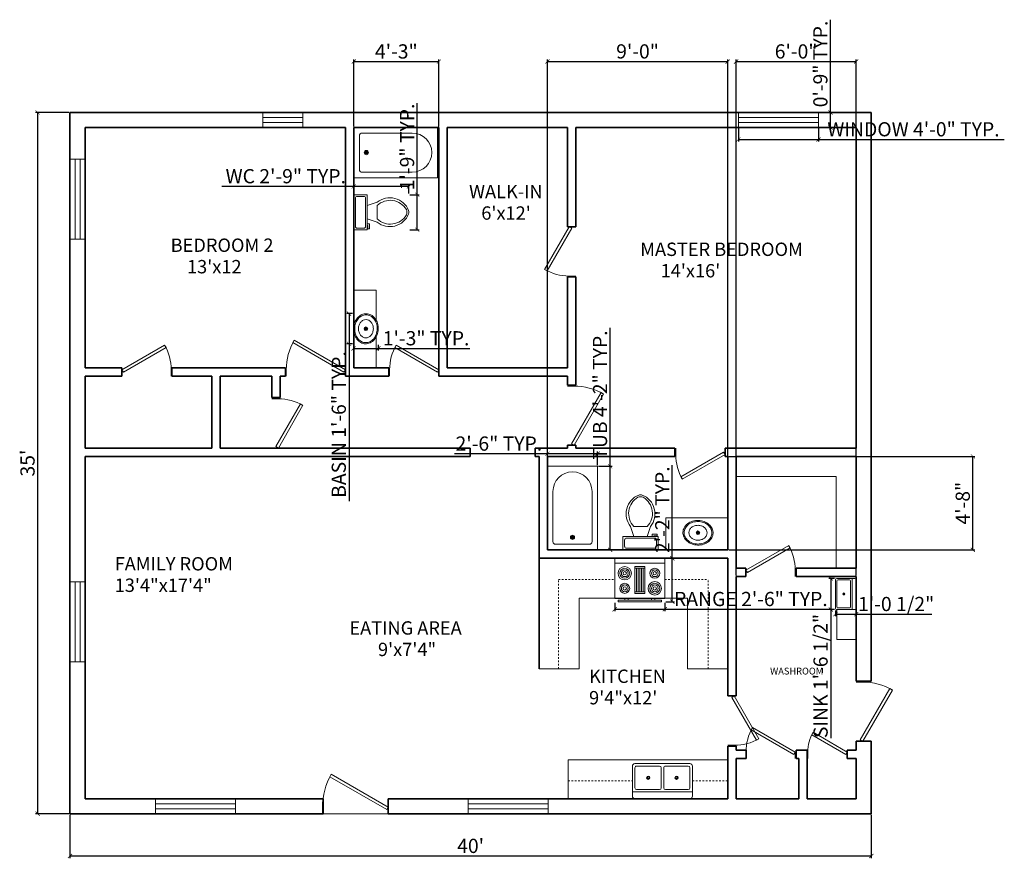
# Model space of a CAD drawing. Units: inches. Extents: x 3799 to 20199, y 1682 to 8087.
# Tile 25 of 30: x 17831 to 18421, y 2751 to 3254. Entities that reach past the tile are written whole.
import ezdxf

# ---------------------------------------------------------------- set-up
doc = ezdxf.new("R2010")
doc.units = ezdxf.units.IN
doc.linetypes.add('JIS_02_1.0', pattern=[2, 1, -1])
for name, color, linetype, lineweight in [('A-ANNO-DIMS', 2, 'Continuous', 18), ('A-AREA-IDEN', 7, 'Continuous', 18), ('A-DOOR', 3, 'Continuous', 18), ('A-EQPM', 9, 'Continuous', 18), ('A-FLOR-CASE', 32, 'Continuous', 18), ('A-FLOR-CASE-OVHD', 32, 'JIS_02_1.0', 13), ('A-FLOR-FIXT', 9, 'Continuous', 18), ('A-FURN', 8, 'Continuous', 18), ('A-GLAZ', 152, 'Continuous', 18), ('A-WALL', 7, 'Continuous', 35)]:
    doc.layers.add(name, color=color, linetype=linetype, lineweight=lineweight)
doc.styles.get("Standard").update_dxf_attribs({"font": 'arial.ttf'})
doc.dimstyles.new('ISO-25', dxfattribs={"dimtxt": 8.5, "dimasz": 2.5, "dimexe": 1.25, "dimexo": 0.625, "dimtad": 1, "dimdec": 0, "dimlunit": 3, "dimtxsty": 'Standard', "dimblk": 'ARCHTICK', "dimcen": 2.5, "dimadec": 0, "dimazin": 0, "dimtfac": 1, "dimtdec": 0, "dimtmove": 0, "dimatfit": 3, "dimfxl": 1, "dimarcsym": 0})

# ---------------------------------------------------------------- blocks, each defined once
blk = doc.blocks.new('*U134')
for p, q in [((0, 0), (0, -100)), ((750, 0), (750, -100))]:
    blk.add_line(p, q)
blk.add_lwpolyline([(0, 0), (650, 375), (671, 337), (22, -38)], close=True)
blk.add_arc((0, 0), 750, 0, 30)
blk = doc.blocks.new('*U135')
for p, q in [((0, 0), (0, -100)), ((-900, 0), (-900, -100))]:
    blk.add_line(p, q)
blk.add_lwpolyline([(0, 0), (-779, 450), (-801, 412), (-22, -38)], close=True)
blk.add_arc((0, 0), 900, 150, 180)
blk = doc.blocks.new('*U136')
for p, q in [((-750, 0), (-750, -100)), ((0, 0), (0, -100))]:
    blk.add_line(p, q)
blk.add_lwpolyline([(0, 0), (-650, 375), (-671, 337), (-22, -38)], close=True)
blk.add_arc((0, 0), 750, 150, 180)
blk = doc.blocks.new('*U141')
for p, q in [((0, 0), (0, -100)), ((750, 0), (750, -100))]:
    blk.add_line(p, q)
blk.add_lwpolyline([(0, 0), (650, 375), (671, 337), (22, -38)], close=True)
blk.add_arc((0, 0), 750, 0, 30)
blk = doc.blocks.new('*U138')
for p, q in [((-750, 0), (-750, 100)), ((0, 0), (0, 100))]:
    blk.add_line(p, q)
blk.add_lwpolyline([(0, 0), (-650, -375), (-671, -337), (-22, 38)], close=True)
blk.add_arc((0, 0), 750, 180, 210)
blk = doc.blocks.new('*U139')
for p, q in [((0, 0), (0, -100)), ((-1000, 0), (-1000, -100))]:
    blk.add_line(p, q)
blk.add_lwpolyline([(0, 0), (-866, 500), (-888, 462), (-22, -38)], close=True)
blk.add_arc((0, 0), 1000, 150, 180)
blk = doc.blocks.new('*U140')
for p, q in [((-750, 0), (-750, -100)), ((0, 0), (0, -100))]:
    blk.add_line(p, q)
blk.add_lwpolyline([(0, 0), (-650, 375), (-671, 337), (-22, -38)], close=True)
blk.add_arc((0, 0), 750, 150, 180)
blk = doc.blocks.new('*U142')
for p, q in [((-600, 0), (-600, -100)), ((0, 0), (0, -100))]:
    blk.add_line(p, q)
blk.add_lwpolyline([(0, 0), (-520, 300), (-541, 262), (-22, -38)], close=True)
blk.add_arc((0, 0), 600, 150, 180)
blk = doc.blocks.new('Bath Tub - 26 x 60 in.')
for p, q in [((8, -18), (10, -18)), ((9, -17), (9, -19))]:
    blk.add_line(p, q)
blk.add_lwpolyline([(0, -36), (0, 0), (60, 0), (60, -36)], close=True)
for points in [[(4, -30), (4, -6)], [(6, -4), (42, -4)], [(42, -32), (6, -32)]]:
    blk.add_lwpolyline(points)
for radius in [1.5, 1]:
    blk.add_circle((9, -18), radius)
for centre, radius, start, end in [((5.75, -5.75), 1.77, 81.8699, 188.1301), ((42, -18), 14, 270, 90), ((5.75, -30.25), 1.77, 171.8699, 278.1301)]:
    blk.add_arc(centre, radius, start, end)
blk = doc.blocks.new('Toilet - top')
for p, q in [((9.5, -6), (9.5, -2)), ((-10, -8.5), (-8, -8.5)), ((-10, -9.5), (-10, -8.5)), ((-7, -9.5), (-10, -9.5)), ((-8, -8.5), (-8, -8)), ((-7, -8), (-7, -9.5)), ((-4, -8), (-6, -14)), ((4, -8), (6, -14)), ((4, -14), (-4, -14))]:
    blk.add_line(p, q)
blk.add_lwpolyline([(10.5, -8), (10.5, 0), (-10.5, 0), (-10.5, -8)], close=True)
for points in [[(-9.5, -2), (-9.5, -6)], [(8.5, -1), (-8.5, -1)], [(-8.5, -7), (8.5, -7)]]:
    blk.add_lwpolyline(points)
for centre, radius, start, end in [((-8.62, -1.88), 0.884, 81.8699, 188.1301), ((8.62, -1.88), 0.884, 351.8699, 98.1301), ((-8.62, -6.12), 0.884, 171.8699, 278.1301), ((8.62, -6.12), 0.884, 261.8699, 8.1301), ((3.52, -21.58), 12.17, 141.46911, 247.97143), ((4.2, -21.82), 11.33, 136.36773, 238.94682), ((-3.52, -21.58), 12.17, 292.02843, 38.53071), ((-4.2, -21.82), 11.33, 301.05301, 43.63209), ((0, -27.88), 4, 245.73182, 294.26817), ((0, -29), 4, 254.86053, 285.13947)]:
    blk.add_arc(centre, radius, start, end)
blk = doc.blocks.new('Sink - Oval top')
for p, q in [((-1, 0), (1, 0)), ((0, 1), (0, -1))]:
    blk.add_line(p, q)
for points in [[(-12.23, 0.39, 0.117634), (-11.46, -3.36, 0.104469), (-8.88, -6.8, 0.090016), (-5.08, -9.07, 0.08192), (-0.32, -10.02, 0.08192), (4.49, -9.38, 0.090016), (8.42, -7.36, 0.104469), (11.22, -4.09, 0.117634), (12.23, -0.39, 0.117634), (11.46, 3.36, 0.104469), (8.88, 6.8, 0.090016), (5.08, 9.07, 0.08192), (0.32, 10.02, 0.08192), (-4.49, 9.38, 0.090016), (-8.42, 7.36, 0.104469), (-11.22, 4.09, 0.117634)], [(-11.29, 0.16, 0.118622), (-10.52, -3.25, 0.104678), (-8.07, -6.36, 0.089562), (-4.54, -8.37, 0.081185), (-0.13, -9.15, 0.081185), (4.3, -8.49, 0.089562), (7.89, -6.58, 0.104678), (10.42, -3.55, 0.118622), (11.29, -0.16, 0.118622), (10.52, 3.25, 0.104678), (8.07, 6.36, 0.089562), (4.54, 8.37, 0.081185), (0.13, 9.15, 0.081185), (-4.3, 8.49, 0.089562), (-7.89, 6.58, 0.104678), (-10.42, 3.55, 0.118622)], [(-7.42, 0.08, 0.118283), (-6.91, -2.17, 0.104607), (-5.29, -4.21, 0.089718), (-2.97, -5.53, 0.081436), (-0.07, -6.04, 0.081436), (2.84, -5.59, 0.089718), (5.2, -4.33, 0.104607), (6.86, -2.32, 0.118283), (7.42, -0.08, 0.118283), (6.91, 2.17, 0.104607), (5.29, 4.21, 0.089718), (2.97, 5.53, 0.081436), (0.07, 6.04, 0.081436), (-2.84, 5.59, 0.089718), (-5.2, 4.33, 0.104607), (-6.86, 2.32, 0.118283)]]:
    blk.add_lwpolyline(points, format="xyb", close=True)
for radius in [1.5, 1]:
    blk.add_circle((0, 0), radius)
blk = doc.blocks.new('Range-Oven - 30 in top')
for p, q in [((0, -3), (30, -3)), ((12, -6), (18, -6)), ((13, -20), (13, -6)), ((14, -6), (14, -20)), ((15, -20), (15, -6)), ((16, -6), (16, -20)), ((17, -20), (17, -6)), ((18, -20), (12, -20)), ((6, -24), (6, -25)), ((8, -25), (8, -24)), ((22, -25), (22, -24)), ((24, -24), (24, -25))]:
    blk.add_line(p, q)
for points in [[(0, -24), (0, 0), (30, 0), (30, -24)], [(12, -21), (12, -5), (18, -5), (18, -21)], [(2, -26), (2, -25), (28, -25), (28, -26)]]:
    blk.add_lwpolyline(points, close=True)
for centre, radius in [((6, -9), 4), ((6, -9), 3), ((6, -9), 2), ((6, -9), 1), ((24, -9), 3), ((24, -9), 2), ((24, -9), 1), ((6, -18), 3), ((6, -18), 2), ((6, -18), 1), ((24, -18), 4), ((24, -18), 3), ((24, -18), 2), ((24, -18), 1)]:
    blk.add_circle(centre, radius)
blk = doc.blocks.new('Sink-double - 36 in top')
for p, q in [((-18, -4), (18, -4)), ((-0.75, -18.5), (-0.75, -6.5)), ((0.75, -6.5), (0.75, -18.5))]:
    blk.add_line(p, q)
for points in [[(-16.5, 0), (16.5, 0)], [(-18, -19.5), (-18, -1.5)], [(-15.5, -5.5), (-1.75, -5.5)], [(1.75, -5.5), (15.5, -5.5)], [(18, -1.5), (18, -19.5)], [(-16.5, -18.5), (-16.5, -6.5)], [(16.5, -6.5), (16.5, -18.5)], [(16.5, -21), (-16.5, -21)], [(-1.75, -19.5), (-15.5, -19.5)], [(15.5, -19.5), (1.75, -19.5)]]:
    blk.add_lwpolyline(points)
for centre, radius in [((-8.5, -12.5), 1), ((8.5, -12.5), 1), ((-8.5, -12.5), 0.5), ((8.5, -12.5), 0.5)]:
    blk.add_circle(centre, radius)
for centre, radius, start, end in [((-16.5, -1.5), 1.5, 90, 180), ((16.5, -1.5), 1.5, 0, 90), ((-15.5, -6.5), 1, 90, 180), ((-1.75, -6.5), 1, 0, 90), ((1.75, -6.5), 1, 90, 180), ((15.5, -6.5), 1, 0, 90), ((-16.5, -19.5), 1.5, 180, 270), ((-15.5, -18.5), 1, 180, 270), ((-1.75, -18.5), 1, 270, 0), ((1.75, -18.5), 1, 180, 270), ((15.5, -18.5), 1, 270, 0), ((16.5, -19.5), 1.5, 270, 0)]:
    blk.add_arc(centre, radius, start, end)
blk = doc.blocks.new('Sink-single - 30 in top')
blk.add_line((-15, -3.999996), (15, -3.999996))
for points in [[(-13.5, 0), (13.5, 0)], [(-15, -18.499996), (-15, -1.5)], [(-13.5, -17.499996), (-13.5, -6.499996)], [(-12.5, -5.499996), (12.5, -5.499996)], [(13.5, -6.499996), (13.5, -17.499996)], [(15, -1.5), (15, -18.499996)], [(12.5, -18.499996), (-12.5, -18.499996)], [(13.5, -19.999996), (-13.5, -19.999996)]]:
    blk.add_lwpolyline(points)
for radius in [1, 0.5]:
    blk.add_circle((0, -11.999996), radius)
for centre, radius, start, end in [((-13.5, -1.5), 1.5, 90, 180), ((-12.5, -6.499996), 1, 90, 180), ((12.5, -6.499996), 1, 0, 90), ((13.5, -1.5), 1.5, 0, 90), ((-13.5, -18.499996), 1.5, 180, 270), ((-12.5, -17.499996), 1, 180, 270), ((12.5, -17.499996), 1, 270, 0), ((13.5, -18.499996), 1.5, 270, 0)]:
    blk.add_arc(centre, radius, start, end)
blk = doc.blocks.new('_ArchTick')
at = {"color": 0, "linetype": 'ByBlock', "const_width": 0.15}
blk.add_lwpolyline([(-0.5, -0.5), (0.5, 0.5)], dxfattribs=at)
blk = doc.blocks.new('*D145')
at = {"layer": 'A-ANNO-DIMS', "color": 0, "lineweight": -2, "transparency": 16777216}
for p, q in [((17861.25, 2777.59), (17861.25, 2751.63)), ((18341.25, 2777.59), (18341.25, 2751.63)), ((17861.25, 2752.88), (18341.25, 2752.88))]:
    blk.add_line(p, q, dxfattribs=at)
at = {"layer": 'Defpoints', "color": 0, "transparency": 16777216}
for p in [(17861.25, 2778.21), (18341.25, 2778.21), (18341.25, 2752.88)]:
    blk.add_point(p, dxfattribs=at)
at = {"layer": 'A-ANNO-DIMS', "color": 0, "lineweight": -2, "transparency": 16777216, "xscale": 2.5, "yscale": 2.5, "zscale": 2.5, "rotation": 180}
blk.add_blockref('_ArchTick', (17861.25, 2752.88), dxfattribs=at)
at = {"layer": 'A-ANNO-DIMS', "color": 0, "lineweight": -2, "transparency": 16777216, "xscale": 2.5, "yscale": 2.5, "zscale": 2.5}
blk.add_blockref('_ArchTick', (18341.25, 2752.88), dxfattribs=at)
at = {"layer": 'A-ANNO-DIMS', "color": 0, "transparency": 16777216, "insert": (18101.25, 2757.84), "char_height": 8.5, "attachment_point": 5}
blk.add_mtext("40'", dxfattribs=at)
blk = doc.blocks.new('*D146')
at = {"layer": 'A-ANNO-DIMS', "color": 0, "lineweight": -2, "transparency": 16777216}
for p, q in [((17860.63, 3198.21), (17840.62, 3198.21)), ((17841.87, 3198.21), (17841.87, 2778.21)), ((17860.63, 2778.21), (17840.62, 2778.21))]:
    blk.add_line(p, q, dxfattribs=at)
at = {"layer": 'Defpoints', "color": 0, "transparency": 16777216}
for p in [(17861.25, 3198.21), (17841.87, 2778.21), (17861.25, 2778.21)]:
    blk.add_point(p, dxfattribs=at)
at = {"layer": 'A-ANNO-DIMS', "color": 0, "lineweight": -2, "transparency": 16777216, "xscale": 2.5, "yscale": 2.5, "zscale": 2.5}
for p, rotation in [((17841.87, 3198.21), 90), ((17841.87, 2778.21), 270)]:
    blk.add_blockref('_ArchTick', p, dxfattribs=dict(at, rotation=rotation))
at = {"layer": 'A-ANNO-DIMS', "color": 0, "transparency": 16777216, "insert": (17836.91, 2988.21), "char_height": 8.5, "attachment_point": 5, "rotation": 90}
blk.add_mtext("35'", dxfattribs=at)
blk = doc.blocks.new('WIN-24IN-9IN-FRAME')
for p, q in [((0, 24), (9, 24)), ((3, 0), (3, 24)), ((6, 0), (6, 24)), ((0, 0), (9, 0))]:
    blk.add_line(p, q)
blk = doc.blocks.new('WIN-48IN-9IN-FRAME')
for p, q in [((0, 0), (0, 9)), ((48, 6), (0, 6)), ((48, 0), (48, 9)), ((48, 3), (0, 3))]:
    blk.add_line(p, q)
blk = doc.blocks.new('*D240')
at = {"layer": 'A-ANNO-DIMS', "color": 0, "lineweight": -2, "transparency": 16777216}
for p, q in [((18261.65, 3188.59), (18261.65, 3180.76)), ((18309.65, 3188.59), (18309.65, 3180.76)), ((18261.65, 3182.01), (18309.65, 3182.01)), ((18309.65, 3182.01), (18420.96, 3182.01))]:
    blk.add_line(p, q, dxfattribs=at)
at = {"layer": 'Defpoints', "color": 0, "transparency": 16777216}
for p in [(18261.65, 3189.21), (18309.65, 3189.21), (18309.65, 3182.01)]:
    blk.add_point(p, dxfattribs=at)
at = {"layer": 'A-ANNO-DIMS', "color": 0, "lineweight": -2, "transparency": 16777216, "xscale": 2.5, "yscale": 2.5, "zscale": 2.5, "rotation": 180}
blk.add_blockref('_ArchTick', (18261.65, 3182.01), dxfattribs=at)
at = {"layer": 'A-ANNO-DIMS', "color": 0, "lineweight": -2, "transparency": 16777216, "xscale": 2.5, "yscale": 2.5, "zscale": 2.5}
blk.add_blockref('_ArchTick', (18309.65, 3182.01), dxfattribs=at)
at = {"layer": 'A-ANNO-DIMS', "color": 0, "transparency": 16777216, "insert": (18366.55, 3187.04), "char_height": 8.5, "attachment_point": 5}
blk.add_mtext('WINDOW 4\'-0" TYP.', dxfattribs=at)
blk = doc.blocks.new('*D241')
at = {"layer": 'A-ANNO-DIMS', "color": 0, "lineweight": -2, "transparency": 16777216}
for p, q in [((18316.85, 3198.21), (18316.85, 3253.77)), ((18310.27, 3198.21), (18318.1, 3198.21)), ((18316.85, 3189.21), (18316.85, 3198.21)), ((18310.27, 3189.21), (18318.1, 3189.21))]:
    blk.add_line(p, q, dxfattribs=at)
at = {"layer": 'Defpoints', "color": 0, "transparency": 16777216}
for p in [(18309.65, 3198.21), (18316.85, 3198.21), (18309.65, 3189.21)]:
    blk.add_point(p, dxfattribs=at)
at = {"layer": 'A-ANNO-DIMS', "color": 0, "lineweight": -2, "transparency": 16777216, "xscale": 2.5, "yscale": 2.5, "zscale": 2.5}
for p, rotation in [((18316.85, 3198.21), 90), ((18316.85, 3189.21), 270)]:
    blk.add_blockref('_ArchTick', p, dxfattribs=dict(at, rotation=rotation))
at = {"layer": 'A-ANNO-DIMS', "color": 0, "transparency": 16777216, "insert": (18311.88, 3227.24), "char_height": 8.5, "attachment_point": 5, "rotation": 90}
blk.add_mtext('0\'-9" TYP.', dxfattribs=at)
blk = doc.blocks.new('*D266')
at = {"layer": 'A-ANNO-DIMS', "color": 0, "lineweight": -2, "transparency": 16777216}
for p, q in [((18031.25, 3153.92), (17952.26, 3153.92)), ((18031.25, 3149.59), (18031.25, 3155.17)), ((18064.3, 3153.92), (18031.25, 3153.92)), ((18064.3, 3149.59), (18064.3, 3155.17))]:
    blk.add_line(p, q, dxfattribs=at)
at = {"layer": 'Defpoints', "color": 0, "transparency": 16777216}
for p in [(18031.25, 3153.92), (18031.25, 3148.96), (18064.3, 3148.96)]:
    blk.add_point(p, dxfattribs=at)
at = {"layer": 'A-ANNO-DIMS', "color": 0, "lineweight": -2, "transparency": 16777216, "xscale": 2.5, "yscale": 2.5, "zscale": 2.5, "rotation": 180}
blk.add_blockref('_ArchTick', (18031.25, 3153.92), dxfattribs=at)
at = {"layer": 'A-ANNO-DIMS', "color": 0, "lineweight": -2, "transparency": 16777216, "xscale": 2.5, "yscale": 2.5, "zscale": 2.5}
blk.add_blockref('_ArchTick', (18064.3, 3153.92), dxfattribs=at)
at = {"layer": 'A-ANNO-DIMS', "color": 0, "transparency": 16777216, "insert": (17990.51, 3158.94), "char_height": 8.5, "attachment_point": 5}
blk.add_mtext('WC 2\'-9" TYP.', dxfattribs=at)
blk = doc.blocks.new('*D267')
at = {"layer": 'A-ANNO-DIMS', "color": 0, "lineweight": -2, "transparency": 16777216}
for p, q in [((18069.26, 3148.96), (18069.26, 3203.72)), ((18064.92, 3148.96), (18070.51, 3148.96)), ((18069.26, 3127.96), (18069.26, 3148.96)), ((18064.92, 3127.96), (18070.51, 3127.96))]:
    blk.add_line(p, q, dxfattribs=at)
at = {"layer": 'Defpoints', "color": 0, "transparency": 16777216}
for p in [(18064.3, 3148.96), (18069.26, 3148.96), (18064.3, 3127.96)]:
    blk.add_point(p, dxfattribs=at)
at = {"layer": 'A-ANNO-DIMS', "color": 0, "lineweight": -2, "transparency": 16777216, "xscale": 2.5, "yscale": 2.5, "zscale": 2.5}
for p, rotation in [((18069.26, 3148.96), 90), ((18069.26, 3127.96), 270)]:
    blk.add_blockref('_ArchTick', p, dxfattribs=dict(at, rotation=rotation))
at = {"layer": 'A-ANNO-DIMS', "color": 0, "transparency": 16777216, "insert": (18064.29, 3177.59), "char_height": 8.5, "attachment_point": 5, "rotation": 90}
blk.add_mtext('1\'-9" TYP.', dxfattribs=at)
blk = doc.blocks.new('*D306')
at = {"layer": 'A-ANNO-DIMS', "color": 0, "lineweight": -2, "transparency": 16777216}
for p, q in [((18184.83, 2986.31), (18184.83, 3069.13)), ((18177.94, 2986.31), (18186.08, 2986.31)), ((18184.83, 2936.21), (18184.83, 2986.31)), ((18177.94, 2936.21), (18186.08, 2936.21))]:
    blk.add_line(p, q, dxfattribs=at)
at = {"layer": 'Defpoints', "color": 0, "transparency": 16777216}
for p in [(18177.31, 2986.31), (18184.83, 2986.31), (18177.31, 2936.21)]:
    blk.add_point(p, dxfattribs=at)
at = {"layer": 'A-ANNO-DIMS', "color": 0, "lineweight": -2, "transparency": 16777216, "xscale": 2.5, "yscale": 2.5, "zscale": 2.5}
for p, rotation in [((18184.83, 2986.31), 90), ((18184.83, 2936.21), 270)]:
    blk.add_blockref('_ArchTick', p, dxfattribs=dict(at, rotation=rotation))
at = {"layer": 'A-ANNO-DIMS', "color": 0, "transparency": 16777216, "insert": (18179.86, 3028.97), "char_height": 8.5, "attachment_point": 5, "rotation": 90}
blk.add_mtext('TUB 4\'-2" TYP.', dxfattribs=at)
blk = doc.blocks.new('*D307')
at = {"layer": 'A-ANNO-DIMS', "color": 0, "lineweight": -2, "transparency": 16777216}
for p, q in [((18147.25, 2993.82), (18091.55, 2993.82)), ((18147.25, 2986.94), (18147.25, 2995.07)), ((18177.31, 2993.82), (18147.25, 2993.82)), ((18177.31, 2986.94), (18177.31, 2995.07))]:
    blk.add_line(p, q, dxfattribs=at)
at = {"layer": 'Defpoints', "color": 0, "transparency": 16777216}
for p in [(18147.25, 2993.82), (18147.25, 2986.31), (18177.31, 2986.31)]:
    blk.add_point(p, dxfattribs=at)
at = {"layer": 'A-ANNO-DIMS', "color": 0, "lineweight": -2, "transparency": 16777216, "xscale": 2.5, "yscale": 2.5, "zscale": 2.5, "rotation": 180}
blk.add_blockref('_ArchTick', (18147.25, 2993.82), dxfattribs=at)
at = {"layer": 'A-ANNO-DIMS', "color": 0, "lineweight": -2, "transparency": 16777216, "xscale": 2.5, "yscale": 2.5, "zscale": 2.5}
blk.add_blockref('_ArchTick', (18177.31, 2993.82), dxfattribs=at)
at = {"layer": 'A-ANNO-DIMS', "color": 0, "transparency": 16777216, "insert": (18118.15, 2998.79), "char_height": 8.5, "attachment_point": 5}
blk.add_mtext('2\'-6" TYP.', dxfattribs=at)
blk = doc.blocks.new('*D314')
at = {"layer": 'A-ANNO-DIMS', "color": 0, "lineweight": -2, "transparency": 16777216}
for p, q in [((18187.56, 2904.57), (18187.56, 2899.44)), ((18217.56, 2904.57), (18217.56, 2899.44)), ((18187.56, 2900.69), (18217.56, 2900.69)), ((18217.56, 2900.69), (18318.21, 2900.69))]:
    blk.add_line(p, q, dxfattribs=at)
at = {"layer": 'Defpoints', "color": 0, "transparency": 16777216}
for p in [(18187.56, 2905.19), (18217.56, 2905.19), (18217.56, 2900.69)]:
    blk.add_point(p, dxfattribs=at)
at = {"layer": 'A-ANNO-DIMS', "color": 0, "lineweight": -2, "transparency": 16777216, "xscale": 2.5, "yscale": 2.5, "zscale": 2.5, "rotation": 180}
blk.add_blockref('_ArchTick', (18187.56, 2900.69), dxfattribs=at)
at = {"layer": 'A-ANNO-DIMS', "color": 0, "lineweight": -2, "transparency": 16777216, "xscale": 2.5, "yscale": 2.5, "zscale": 2.5}
blk.add_blockref('_ArchTick', (18217.56, 2900.69), dxfattribs=at)
at = {"layer": 'A-ANNO-DIMS', "color": 0, "transparency": 16777216, "insert": (18269.13, 2905.71), "char_height": 8.5, "attachment_point": 5}
blk.add_mtext('RANGE 2\'-6" TYP.', dxfattribs=at)
blk = doc.blocks.new('*D315')
at = {"layer": 'A-ANNO-DIMS', "color": 0, "lineweight": -2, "transparency": 16777216}
for p, q in [((18222.06, 2931.19), (18222.06, 2986.9)), ((18218.18, 2931.19), (18223.31, 2931.19)), ((18222.06, 2905.19), (18222.06, 2931.19)), ((18218.18, 2905.19), (18223.31, 2905.19))]:
    blk.add_line(p, q, dxfattribs=at)
at = {"layer": 'Defpoints', "color": 0, "transparency": 16777216}
for p in [(18217.56, 2931.19), (18222.06, 2931.19), (18217.56, 2905.19)]:
    blk.add_point(p, dxfattribs=at)
at = {"layer": 'A-ANNO-DIMS', "color": 0, "lineweight": -2, "transparency": 16777216, "xscale": 2.5, "yscale": 2.5, "zscale": 2.5}
for p, rotation in [((18222.06, 2931.19), 90), ((18222.06, 2905.19), 270)]:
    blk.add_blockref('_ArchTick', p, dxfattribs=dict(at, rotation=rotation))
at = {"layer": 'A-ANNO-DIMS', "color": 0, "transparency": 16777216, "insert": (18217.16, 2960.29), "char_height": 8.5, "attachment_point": 5, "rotation": 90}
blk.add_mtext('2\'-2" TYP.', dxfattribs=at)
blk = doc.blocks.new('*D322')
at = {"layer": 'A-ANNO-DIMS', "color": 0, "lineweight": -2, "transparency": 16777216}
for p, q in [((18319.17, 2919.18), (18315.75, 2919.18)), ((18317, 2919.18), (18317, 2900.49)), ((18319.17, 2900.49), (18315.75, 2900.49)), ((18317, 2900.49), (18317, 2823.37))]:
    blk.add_line(p, q, dxfattribs=at)
at = {"layer": 'Defpoints', "color": 0, "transparency": 16777216}
for p in [(18319.8, 2919.18), (18317, 2900.49), (18319.8, 2900.49)]:
    blk.add_point(p, dxfattribs=at)
at = {"layer": 'A-ANNO-DIMS', "color": 0, "lineweight": -2, "transparency": 16777216, "xscale": 2.5, "yscale": 2.5, "zscale": 2.5}
for p, rotation in [((18317, 2919.18), 90), ((18317, 2900.49), 270)]:
    blk.add_blockref('_ArchTick', p, dxfattribs=dict(at, rotation=rotation))
at = {"layer": 'A-ANNO-DIMS', "color": 0, "transparency": 16777216, "insert": (18311.98, 2860.68), "char_height": 8.5, "attachment_point": 5, "rotation": 90}
blk.add_mtext('SINK 1\'-6 1/2"', dxfattribs=at)
blk = doc.blocks.new('*D323')
at = {"layer": 'A-ANNO-DIMS', "color": 0, "lineweight": -2, "transparency": 16777216}
for p, q in [((18319.8, 2899.87), (18319.8, 2896.44)), ((18319.8, 2897.69), (18332.25, 2897.69)), ((18332.25, 2899.87), (18332.25, 2896.44)), ((18332.25, 2897.69), (18377.6, 2897.69))]:
    blk.add_line(p, q, dxfattribs=at)
at = {"layer": 'Defpoints', "color": 0, "transparency": 16777216}
for p in [(18319.8, 2900.49), (18332.25, 2900.49), (18332.25, 2897.69)]:
    blk.add_point(p, dxfattribs=at)
at = {"layer": 'A-ANNO-DIMS', "color": 0, "lineweight": -2, "transparency": 16777216, "xscale": 2.5, "yscale": 2.5, "zscale": 2.5, "rotation": 180}
blk.add_blockref('_ArchTick', (18319.8, 2897.69), dxfattribs=at)
at = {"layer": 'A-ANNO-DIMS', "color": 0, "lineweight": -2, "transparency": 16777216, "xscale": 2.5, "yscale": 2.5, "zscale": 2.5}
blk.add_blockref('_ArchTick', (18332.25, 2897.69), dxfattribs=at)
at = {"layer": 'A-ANNO-DIMS', "color": 0, "transparency": 16777216, "insert": (18356.18, 2902.71), "char_height": 8.5, "attachment_point": 5}
blk.add_mtext('1\'-0 1/2"', dxfattribs=at)
blk = doc.blocks.new('*D334')
at = {"layer": 'A-ANNO-DIMS', "color": 0, "lineweight": -2, "transparency": 16777216}
for p, q in [((18030.48, 3077.72), (18027.14, 3077.72)), ((18028.39, 3077.72), (18028.39, 3059.62)), ((18030.48, 3059.62), (18027.14, 3059.62)), ((18028.39, 3059.62), (18028.39, 2965.5))]:
    blk.add_line(p, q, dxfattribs=at)
at = {"layer": 'Defpoints', "color": 0, "transparency": 16777216}
for p in [(18031.1, 3077.72), (18028.39, 3059.62), (18031.1, 3059.62)]:
    blk.add_point(p, dxfattribs=at)
at = {"layer": 'A-ANNO-DIMS', "color": 0, "lineweight": -2, "transparency": 16777216, "xscale": 2.5, "yscale": 2.5, "zscale": 2.5}
for p, rotation in [((18028.39, 3077.72), 90), ((18028.39, 3059.62), 270)]:
    blk.add_blockref('_ArchTick', p, dxfattribs=dict(at, rotation=rotation))
at = {"layer": 'A-ANNO-DIMS', "color": 0, "transparency": 16777216, "insert": (18023.37, 3011.31), "char_height": 8.5, "attachment_point": 5, "rotation": 90}
blk.add_mtext('BASIN 1\'-6" TYP.', dxfattribs=at)
blk = doc.blocks.new('*D335')
at = {"layer": 'A-ANNO-DIMS', "color": 0, "lineweight": -2, "transparency": 16777216}
for p, q in [((18031.1, 3058.99), (18031.1, 3055.65)), ((18031.1, 3056.9), (18045.95, 3056.9)), ((18045.95, 3058.99), (18045.95, 3055.65)), ((18045.95, 3056.9), (18100.71, 3056.9))]:
    blk.add_line(p, q, dxfattribs=at)
at = {"layer": 'Defpoints', "color": 0, "transparency": 16777216}
for p in [(18031.1, 3059.62), (18045.95, 3059.62), (18045.95, 3056.9)]:
    blk.add_point(p, dxfattribs=at)
at = {"layer": 'A-ANNO-DIMS', "color": 0, "lineweight": -2, "transparency": 16777216, "xscale": 2.5, "yscale": 2.5, "zscale": 2.5, "rotation": 180}
blk.add_blockref('_ArchTick', (18031.1, 3056.9), dxfattribs=at)
at = {"layer": 'A-ANNO-DIMS', "color": 0, "lineweight": -2, "transparency": 16777216, "xscale": 2.5, "yscale": 2.5, "zscale": 2.5}
blk.add_blockref('_ArchTick', (18045.95, 3056.9), dxfattribs=at)
at = {"layer": 'A-ANNO-DIMS', "color": 0, "transparency": 16777216, "insert": (18074.58, 3061.87), "char_height": 8.5, "attachment_point": 5}
blk.add_mtext('1\'-3" TYP.', dxfattribs=at)
blk = doc.blocks.new('*D375')
at = {"layer": 'A-ANNO-DIMS', "color": 0, "lineweight": -2, "transparency": 16777216}
for p, q in [((18031.25, 3189.84), (18031.25, 3229.96)), ((18031.25, 3228.71), (18082.25, 3228.71)), ((18082.25, 3189.84), (18082.25, 3229.96))]:
    blk.add_line(p, q, dxfattribs=at)
at = {"layer": 'Defpoints', "color": 0, "transparency": 16777216}
for p in [(18082.25, 3228.71), (18031.25, 3189.21), (18082.25, 3189.21)]:
    blk.add_point(p, dxfattribs=at)
at = {"layer": 'A-ANNO-DIMS', "color": 0, "lineweight": -2, "transparency": 16777216, "xscale": 2.5, "yscale": 2.5, "zscale": 2.5, "rotation": 180}
blk.add_blockref('_ArchTick', (18031.25, 3228.71), dxfattribs=at)
at = {"layer": 'A-ANNO-DIMS', "color": 0, "lineweight": -2, "transparency": 16777216, "xscale": 2.5, "yscale": 2.5, "zscale": 2.5}
blk.add_blockref('_ArchTick', (18082.25, 3228.71), dxfattribs=at)
at = {"layer": 'A-ANNO-DIMS', "color": 0, "transparency": 16777216, "insert": (18056.75, 3233.68), "char_height": 8.5, "attachment_point": 5}
blk.add_mtext('4\'-3"', dxfattribs=at)
blk = doc.blocks.new('*D376')
at = {"layer": 'A-ANNO-DIMS', "color": 0, "lineweight": -2, "transparency": 16777216}
for p, q in [((18147.25, 2936.84), (18147.25, 3229.96)), ((18147.25, 3228.71), (18255.25, 3228.71)), ((18255.25, 2936.84), (18255.25, 3229.96))]:
    blk.add_line(p, q, dxfattribs=at)
at = {"layer": 'Defpoints', "color": 0, "transparency": 16777216}
for p in [(18255.25, 3228.71), (18147.25, 2936.21), (18255.25, 2936.21)]:
    blk.add_point(p, dxfattribs=at)
at = {"layer": 'A-ANNO-DIMS', "color": 0, "lineweight": -2, "transparency": 16777216, "xscale": 2.5, "yscale": 2.5, "zscale": 2.5, "rotation": 180}
blk.add_blockref('_ArchTick', (18147.25, 3228.71), dxfattribs=at)
at = {"layer": 'A-ANNO-DIMS', "color": 0, "lineweight": -2, "transparency": 16777216, "xscale": 2.5, "yscale": 2.5, "zscale": 2.5}
blk.add_blockref('_ArchTick', (18255.25, 3228.71), dxfattribs=at)
at = {"layer": 'A-ANNO-DIMS', "color": 0, "transparency": 16777216, "insert": (18201.25, 3233.68), "char_height": 8.5, "attachment_point": 5}
blk.add_mtext('9\'-0"', dxfattribs=at)
blk = doc.blocks.new('*D377')
at = {"layer": 'A-ANNO-DIMS', "color": 0, "lineweight": -2, "transparency": 16777216}
for p, q in [((18255.88, 2992.21), (18403.37, 2992.21)), ((18402.12, 2936.21), (18402.12, 2992.21)), ((18255.88, 2936.21), (18403.37, 2936.21))]:
    blk.add_line(p, q, dxfattribs=at)
at = {"layer": 'Defpoints', "color": 0, "transparency": 16777216}
for p in [(18255.25, 2992.21), (18402.12, 2992.21), (18255.25, 2936.21)]:
    blk.add_point(p, dxfattribs=at)
at = {"layer": 'A-ANNO-DIMS', "color": 0, "lineweight": -2, "transparency": 16777216, "xscale": 2.5, "yscale": 2.5, "zscale": 2.5}
for p, rotation in [((18402.12, 2992.21), 90), ((18402.12, 2936.21), 270)]:
    blk.add_blockref('_ArchTick', p, dxfattribs=dict(at, rotation=rotation))
at = {"layer": 'A-ANNO-DIMS', "color": 0, "transparency": 16777216, "insert": (18397.16, 2964.21), "char_height": 8.5, "attachment_point": 5, "rotation": 90}
blk.add_mtext('4\'-8"', dxfattribs=at)
blk = doc.blocks.new('*D378')
at = {"layer": 'A-ANNO-DIMS', "color": 0, "lineweight": -2, "transparency": 16777216}
for p, q in [((18260.25, 2920.84), (18260.25, 3229.96)), ((18260.25, 3228.71), (18332.25, 3228.71)), ((18332.25, 2920.84), (18332.25, 3229.96))]:
    blk.add_line(p, q, dxfattribs=at)
at = {"layer": 'Defpoints', "color": 0, "transparency": 16777216}
for p in [(18332.25, 3228.71), (18260.25, 2920.21), (18332.25, 2920.21)]:
    blk.add_point(p, dxfattribs=at)
at = {"layer": 'A-ANNO-DIMS', "color": 0, "lineweight": -2, "transparency": 16777216, "xscale": 2.5, "yscale": 2.5, "zscale": 2.5, "rotation": 180}
blk.add_blockref('_ArchTick', (18260.25, 3228.71), dxfattribs=at)
at = {"layer": 'A-ANNO-DIMS', "color": 0, "lineweight": -2, "transparency": 16777216, "xscale": 2.5, "yscale": 2.5, "zscale": 2.5}
blk.add_blockref('_ArchTick', (18332.25, 3228.71), dxfattribs=at)
at = {"layer": 'A-ANNO-DIMS', "color": 0, "transparency": 16777216, "insert": (18296.25, 3233.68), "char_height": 8.5, "attachment_point": 5}
blk.add_mtext('6\'-0"', dxfattribs=at)

msp = doc.modelspace()

# ---------------------------------------------------------------- linework, layer by layer
at = {"layer": 'A-DOOR'}
msp.add_line((18051.86, 2778.21), (18012.86, 2778.21), dxfattribs=at)
at = {"layer": 'A-FLOR-CASE'}
for p, q in [((18044.74, 3091.72), (18031.25, 3091.72)), ((18044.74, 3073.66), (18044.74, 3091.72)), ((18044.74, 3045.21), (18044.74, 3063.87)), ((18320.25, 2980.21), (18260.25, 2980.21)), ((18320.25, 2925.21), (18320.25, 2980.21)), ((18255.25, 2955.42), (18218.18, 2955.42)), ((18218.18, 2955.42), (18218.18, 2936.21)), ((18166.25, 2907.21), (18231.25, 2907.21)), ((18166.25, 2864.9), (18166.25, 2907.21)), ((18231.25, 2864.9), (18231.25, 2907.21)), ((18142.25, 2864.9), (18166.25, 2864.9)), ((18231.25, 2864.9), (18255.25, 2864.9)), ((18255.25, 2810.39), (18159.6, 2810.39)), ((18159.6, 2810.39), (18159.6, 2787.21))]:
    msp.add_line(p, q, dxfattribs=at)
at = {"layer": 'A-FLOR-CASE-OVHD'}
for p, q in [((18153.93, 2864.9), (18153.93, 2918.41)), ((18153.93, 2918.41), (18187.56, 2918.41)), ((18217.56, 2918.41), (18243.65, 2918.41)), ((18243.65, 2864.9), (18243.65, 2918.41)), ((18159.6, 2797.89), (18198.15, 2797.89)), ((18234.15, 2797.89), (18255.25, 2797.89))]:
    msp.add_line(p, q, dxfattribs=at)
at = {"layer": 'A-FURN'}
msp.add_lwpolyline([(18320.73, 2900.49), (18332.25, 2900.49), (18332.25, 2882.64), (18320.73, 2882.64)], close=True, dxfattribs=at)
at = {"layer": 'A-WALL'}
for p, q in [((18341.25, 3198.21), (17861.25, 3198.21)), ((17861.25, 3198.21), (17861.25, 2778.21)), ((18341.25, 2857.63), (18341.25, 3198.21)), ((17870.25, 3189.21), (17870.25, 3045.21)), ((18026.25, 3189.21), (17870.25, 3189.21)), ((18026.25, 3189.21), (18026.25, 3040.21)), ((18031.25, 3189.21), (18031.25, 3045.21)), ((18082.25, 3189.21), (18031.25, 3189.21)), ((18082.25, 3045.21), (18082.25, 3189.21)), ((18087.25, 3045.21), (18087.25, 3189.21)), ((18159.25, 3189.21), (18087.25, 3189.21)), ((18159.25, 3129.75), (18159.25, 3189.21)), ((18332.25, 3189.21), (18164.25, 3189.21)), ((18164.25, 3129.75), (18164.25, 3189.21)), ((18332.25, 2997.21), (18332.25, 3189.21)), ((18164.25, 3129.75), (18159.25, 3129.75)), ((18159.25, 3045.21), (18159.25, 3099.75)), ((18164.25, 3099.75), (18159.25, 3099.75)), ((18164.25, 3034.9), (18164.25, 3099.75)), ((17892.35, 3045.21), (17870.25, 3045.21)), ((17892.35, 3040.21), (17892.35, 3045.21)), ((17990.25, 3045.21), (17922.35, 3045.21)), ((17922.35, 3040.21), (17922.35, 3045.21)), ((17990.25, 3045.21), (17990.25, 3040.21)), ((18052.25, 3045.21), (18031.25, 3045.21)), ((18052.25, 3045.21), (18052.25, 3040.21)), ((18082.25, 3045.21), (18082.25, 3040.21)), ((18159.25, 3045.21), (18087.25, 3045.21)), ((17870.25, 3040.21), (17870.25, 2997.21)), ((17892.35, 3040.21), (17870.25, 3040.21)), ((17946.13, 3040.21), (17922.35, 3040.21)), ((17946.13, 3040.21), (17946.13, 2997.21)), ((17982.13, 3040.21), (17951.13, 3040.21)), ((17951.13, 3040.21), (17951.13, 2997.21)), ((17982.13, 3040.21), (17982.13, 3027.4)), ((17990.25, 3040.21), (17987.13, 3040.21)), ((17987.13, 3040.21), (17987.13, 3027.4)), ((18052.25, 3040.21), (18026.25, 3040.21)), ((18159.25, 3040.21), (18082.25, 3040.21)), ((18159.25, 3034.9), (18159.25, 3040.21)), ((18159.25, 3034.9), (18164.25, 3034.9)), ((17982.13, 3027.4), (17987.13, 3027.4)), ((17946.13, 2997.21), (17870.25, 2997.21)), ((18100.96, 2997.21), (17951.13, 2997.21)), ((18100.96, 2992.21), (18100.96, 2997.21)), ((18159.25, 2997.21), (18139.96, 2997.21)), ((18139.96, 2992.21), (18139.96, 2997.21)), ((18159.25, 2997.21), (18159.25, 2998.9)), ((18159.25, 2998.9), (18164.25, 2998.9)), ((18164.25, 2997.21), (18164.25, 2998.9)), ((18223.65, 2997.21), (18164.25, 2997.21)), ((18223.65, 2992.21), (18223.65, 2997.21)), ((18332.25, 2997.21), (18253.65, 2997.21)), ((18253.65, 2992.21), (18253.65, 2997.21)), ((17870.25, 2992.21), (17870.25, 2787.21)), ((18100.96, 2992.21), (17870.25, 2992.21)), ((18142.25, 2992.21), (18139.96, 2992.21)), ((18142.25, 2864.9), (18142.25, 2992.21)), ((18164.25, 2992.21), (18147.25, 2992.21)), ((18147.25, 2936.21), (18147.25, 2992.21)), ((18223.65, 2992.21), (18159.25, 2992.21)), ((18255.25, 2992.21), (18253.65, 2992.21)), ((18255.25, 2936.21), (18255.25, 2992.21)), ((18332.25, 2992.21), (18260.25, 2992.21)), ((18260.25, 2925.21), (18260.25, 2992.21)), ((18332.25, 2925.21), (18332.25, 2992.21)), ((18147.25, 2936.21), (18255.25, 2936.21)), ((18142.25, 2931.21), (18255.25, 2931.21)), ((18255.25, 2848.71), (18255.25, 2931.21)), ((18266.19, 2925.21), (18260.25, 2925.21)), ((18260.25, 2848.71), (18260.25, 2920.21)), ((18266.19, 2920.21), (18260.25, 2920.21)), ((18266.19, 2925.21), (18266.19, 2920.21)), ((18332.25, 2925.21), (18296.19, 2925.21)), ((18296.19, 2925.21), (18296.19, 2920.21)), ((18332.25, 2920.21), (18296.19, 2920.21)), ((18332.25, 2857.63), (18332.25, 2920.21)), ((18332.25, 2857.63), (18341.25, 2857.63)), ((18260.25, 2848.71), (18255.25, 2848.71)), ((18332.25, 2816.21), (18332.25, 2821.63)), ((18332.25, 2821.63), (18341.25, 2821.63)), ((18341.25, 2778.21), (18341.25, 2821.63)), ((18255.25, 2787.21), (18255.25, 2818.71)), ((18260.25, 2818.71), (18255.25, 2818.71)), ((18260.25, 2816.21), (18260.25, 2818.71)), ((18260.25, 2816.21), (18266.23, 2816.21)), ((18266.23, 2811.21), (18266.23, 2816.21)), ((18296.23, 2811.21), (18296.23, 2816.21)), ((18296.23, 2816.21), (18302.81, 2816.21)), ((18302.81, 2811.21), (18302.81, 2816.21)), ((18326.81, 2811.21), (18326.81, 2816.21)), ((18326.81, 2816.21), (18332.25, 2816.21)), ((18260.25, 2787.21), (18260.25, 2811.21)), ((18260.25, 2811.21), (18266.23, 2811.21)), ((18296.23, 2811.21), (18297.81, 2811.21)), ((18297.81, 2811.21), (18297.81, 2787.21)), ((18302.81, 2811.21), (18302.81, 2787.21)), ((18326.81, 2811.21), (18332.25, 2811.21)), ((18332.25, 2787.21), (18332.25, 2811.21)), ((17870.25, 2787.21), (18012.86, 2787.21)), ((18012.86, 2787.21), (18012.86, 2778.21)), ((18051.86, 2787.21), (18051.86, 2778.21)), ((18051.86, 2787.21), (18255.25, 2787.21)), ((18260.25, 2787.21), (18297.81, 2787.21)), ((18302.81, 2787.21), (18332.25, 2787.21)), ((17861.25, 2778.21), (18012.86, 2778.21)), ((18051.86, 2778.21), (18341.25, 2778.21))]:
    msp.add_line(p, q, dxfattribs=at)

# ---------------------------------------------------------------- block references
at = {"layer": 'A-DOOR', "xscale": 0.0393700787401575, "yscale": 0.0393700787401575, "zscale": 0.0393700787401575}
for name, p, rotation in [('*U136', (18160.32, 3129.75), 90), ('*U135', (18163.19, 2998.9), 270), ('*U136', (17986.06, 2997.21), 270), ('*U135', (18336.19, 2821.63), 270), ('*U141', (18259.19, 2848.71), 270)]:
    msp.add_blockref(name, p, dxfattribs=dict(at, rotation=rotation))
for name, p in [('*U135', (18026.25, 3044.15)), ('*U134', (17892.35, 3044.15)), ('*U136', (18082.25, 3044.15)), ('*U138', (18253.65, 2993.28)), ('*U134', (18266.19, 2924.15)), ('*U140', (18295.76, 2815.15)), ('*U142', (18326.9, 2815.15)), ('*U139', (18051.86, 2782.15))]:
    msp.add_blockref(name, p, dxfattribs=at)
at = {"layer": 'A-EQPM'}
msp.add_blockref('Range-Oven - 30 in top', (18187.56, 2931.19), dxfattribs=at)
at = {"layer": 'A-FLOR-FIXT'}
for name, p, xscale, yscale, zscale in [('Bath Tub - 26 x 60 in.', (18031.25, 3189.21), 0.8349521512078489, 0.8349521512078489, 0.8349521512078489), ('Sink - Oval top', (18237.46, 2946.48), 0.7371812533597285, 0.7371812533597285, 0.7371812533597285)]:
    msp.add_blockref(name, p, dxfattribs=dict(at, xscale=xscale, yscale=yscale, zscale=zscale))
for name, p, rotation in [('Toilet - top', (18031.25, 3138.46), 90), ('Toilet - top', (18203.03, 2936.21), 180), ('Sink-double - 36 in top', (18216.15, 2787.21), 180)]:
    msp.add_blockref(name, p, dxfattribs=dict(at, rotation=rotation))
for name, p, xscale, yscale, zscale, rotation in [('Sink - Oval top', (18038.53, 3068.67), 0.7371812533597285, 0.7371812533597285, 0.7371812533597285, 270), ('Bath Tub - 26 x 60 in.', (18147.25, 2936.21), 0.8349521512078489, 0.8349521512078489, 0.8349521512078489, 90), ('Sink-single - 30 in top', (18332.25, 2909.83), 0.622792348153793, 0.622792348153793, 0.622792348153793, 270)]:
    msp.add_blockref(name, p, dxfattribs=dict(at, xscale=xscale, yscale=yscale, zscale=zscale, rotation=rotation))
at = {"layer": 'A-GLAZ', "rotation": 90}
for name, p in [('WIN-24IN-9IN-FRAME', (18000.8, 3189.21)), ('WIN-48IN-9IN-FRAME', (17870.25, 3122.24)), ('WIN-48IN-9IN-FRAME', (17870.25, 2869.13))]:
    msp.add_blockref(name, p, dxfattribs=at)
at = {"layer": 'A-GLAZ'}
for p in [(18261.65, 3189.21), (17912.49, 2778.21), (18099.76, 2778.21)]:
    msp.add_blockref('WIN-48IN-9IN-FRAME', p, dxfattribs=at)

# ---------------------------------------------------------------- texts
at = {"layer": 'A-AREA-IDEN'}
for s, height, p in [('WALK-IN', 8, (18100.3, 3146.83)), ("   6'x12'", 8, (18100.31, 3133.98)), ('BEDROOM 2', 8, (17921.55, 3114.7)), ('MASTER BEDROOM', 8, (18202.84, 3112.26)), ("    13'x12", 8, (17921.55, 3101.85)), ("     14'x16'", 8, (18202.84, 3099.41)), ('FAMILY ROOM', 8, (17888.01, 2923.88)), ('13\'4"x17\'4"', 8, (17888.01, 2911.03)), ('EATING AREA', 8, (18028.64, 2885.46)), ('       9\'x7\'4"', 8, (18028.64, 2872.6)), ('KITCHEN', 8, (18172.21, 2856.53)), ('WASHROOM', 4.067, (18280.66, 2861.58)), ('9\'4"x12\'', 8, (18172.21, 2843.68))]:
    msp.add_text(s, height=height, rotation=0.00222, dxfattribs=at).set_placement(p)

# ---------------------------------------------------------------- dimensions: what is measured, and where the dimension line sits
at = {"layer": 'A-ANNO-DIMS'}
for base, p1, p2, angle, text, picture, middle in [((18316.85, 3198.21), (18309.65, 3189.21), (18309.65, 3198.21), 90, '<> TYP.', '*D241', (18311.88, 3227.24)), ((18069.26, 3148.96), (18064.3, 3127.96), (18064.3, 3148.96), 90, '<> TYP.', '*D267', (18064.29, 3177.59)), ((18031.2536, 3153.9203), (18064.2998, 3148.9634), (18031.2536, 3148.9634), 180, 'WC <> TYP.', '*D266', (17990.5077, 3158.9403)), ((18028.39, 3059.62), (18031.1, 3077.72), (18031.1, 3059.62), 270, 'BASIN <> TYP.', '*D334', (18023.37, 3011.31)), ((18184.83, 2986.31), (18177.31, 2936.21), (18177.31, 2986.31), 90, 'TUB <> TYP.', '*D306', (18179.86, 3028.97)), ((18147.25, 2993.82), (18177.31, 2986.31), (18147.25, 2986.31), 180, '<> TYP.', '*D307', (18118.15, 2998.79)), ((18222.06, 2931.19), (18217.56, 2905.19), (18217.56, 2931.19), 90, '<> TYP.', '*D315', (18217.16, 2960.29)), ((18317, 2900.49), (18319.8, 2919.18), (18319.8, 2900.49), 270, 'SINK <>', '*D322', (18311.98, 2860.68))]:
    dim = msp.add_linear_dim(base=base, p1=p1, p2=p2, angle=angle, text=text, dimstyle='ISO-25', override={"dimdec": 1, "dimlfac": 1, "dimrnd": 0, "dimzin": 1, "dimdsep": 46, "dimlunit": 4, "dimfrac": 2}, dxfattribs=at)
    dim.commit()
    dim.dimension.update_dxf_attribs({"geometry": picture, "text_midpoint": middle})
for base, p1, p2, override, picture, middle in [((18082.25, 3228.71), (18031.25, 3189.21), (18082.25, 3189.21), {"dimdec": 1, "dimlfac": 1, "dimrnd": 0, "dimzin": 1, "dimdsep": 46, "dimlunit": 4, "dimfrac": 2}, '*D375', (18056.75, 3233.68)), ((18255.25, 3228.71), (18147.25, 2936.21), (18255.25, 2936.21), {"dimdec": 1, "dimlfac": 1, "dimrnd": 0, "dimzin": 1, "dimdsep": 46, "dimlunit": 4, "dimfrac": 2}, '*D376', (18201.25, 3233.68)), ((18332.25, 3228.71), (18260.25, 2920.21), (18332.25, 2920.21), {"dimdec": 1, "dimlfac": 1, "dimrnd": 0, "dimzin": 1, "dimdsep": 46, "dimlunit": 4, "dimfrac": 2}, '*D378', (18296.25, 3233.68)), ((18332.2536, 2897.6891), (18319.7978, 2900.4917), (18332.2536, 2900.4917), {"dimdec": 1, "dimlfac": 1, "dimrnd": 0, "dimzin": 1, "dimdsep": 46, "dimlunit": 4, "dimfrac": 2}, '*D323', (18356.1793, 2902.7091)), ((18341.25, 2752.88), (17861.25, 2778.21), (18341.25, 2778.21), {"dimclrd": 0, "dimclre": 0, "dimclrt": 0}, '*D145', (18101.25, 2757.84))]:
    dim = msp.add_linear_dim(base=base, p1=p1, p2=p2, dimstyle='ISO-25', override=override, dxfattribs=at)
    dim.commit()
    dim.dimension.update_dxf_attribs({"geometry": picture, "text_midpoint": middle})
for base, p1, p2, text, picture, middle in [((18309.65, 3182.01), (18261.65, 3189.21), (18309.65, 3189.21), 'WINDOW <> TYP.', '*D240', (18366.55, 3187.04)), ((18045.9487, 3056.902), (18031.1044, 3059.6167), (18045.9487, 3059.6167), '<> TYP.', '*D335', (18074.5795, 3061.8697)), ((18217.56, 2900.69), (18187.56, 2905.19), (18217.56, 2905.19), 'RANGE <> TYP.', '*D314', (18269.13, 2905.71))]:
    dim = msp.add_linear_dim(base=base, p1=p1, p2=p2, text=text, dimstyle='ISO-25', override={"dimdec": 1, "dimlfac": 1, "dimrnd": 0, "dimzin": 1, "dimdsep": 46, "dimlunit": 4, "dimfrac": 2}, dxfattribs=at)
    dim.commit()
    dim.dimension.update_dxf_attribs({"geometry": picture, "text_midpoint": middle})
for base, p1, p2, override, picture, middle in [((17841.87, 2778.21), (17861.25, 3198.21), (17861.25, 2778.21), {"dimclrd": 0, "dimclre": 0, "dimclrt": 0}, '*D146', (17836.91, 2988.21)), ((18402.12, 2992.21), (18255.25, 2936.21), (18255.25, 2992.21), {"dimdec": 1, "dimlfac": 1, "dimrnd": 0, "dimzin": 1, "dimdsep": 46, "dimlunit": 4, "dimfrac": 2}, '*D377', (18397.16, 2964.21))]:
    dim = msp.add_linear_dim(base=base, p1=p1, p2=p2, angle=90, dimstyle='ISO-25', override=override, dxfattribs=at)
    dim.commit()
    dim.dimension.update_dxf_attribs({"geometry": picture, "text_midpoint": middle})

doc.saveas('drawing.dxf')
